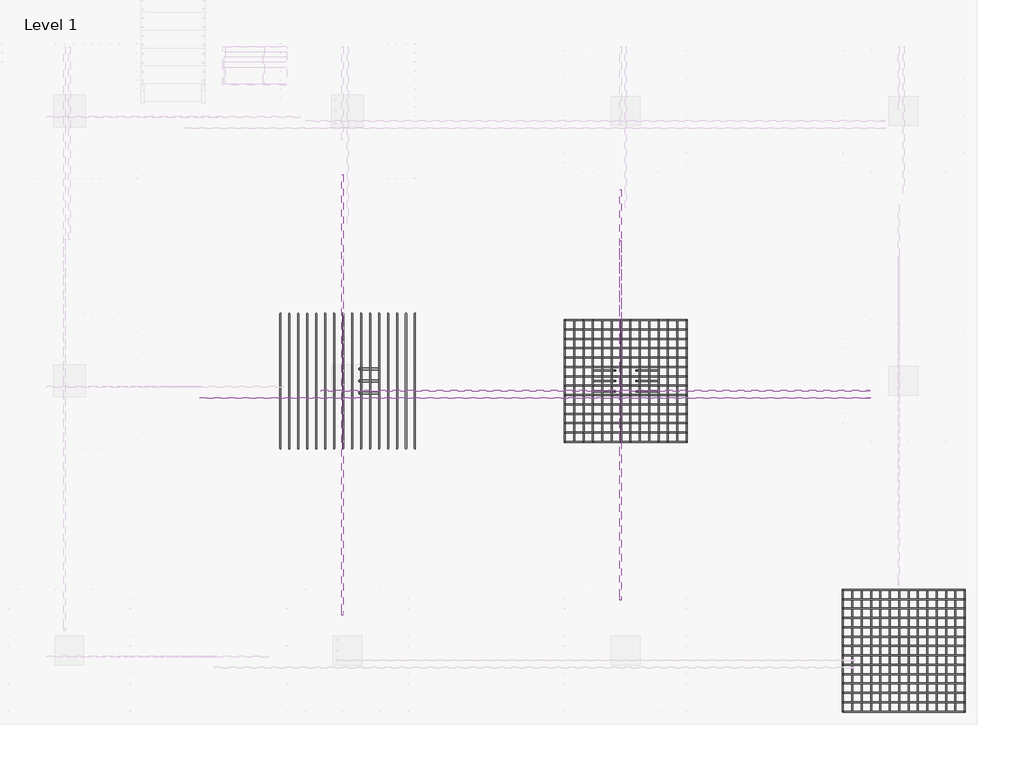
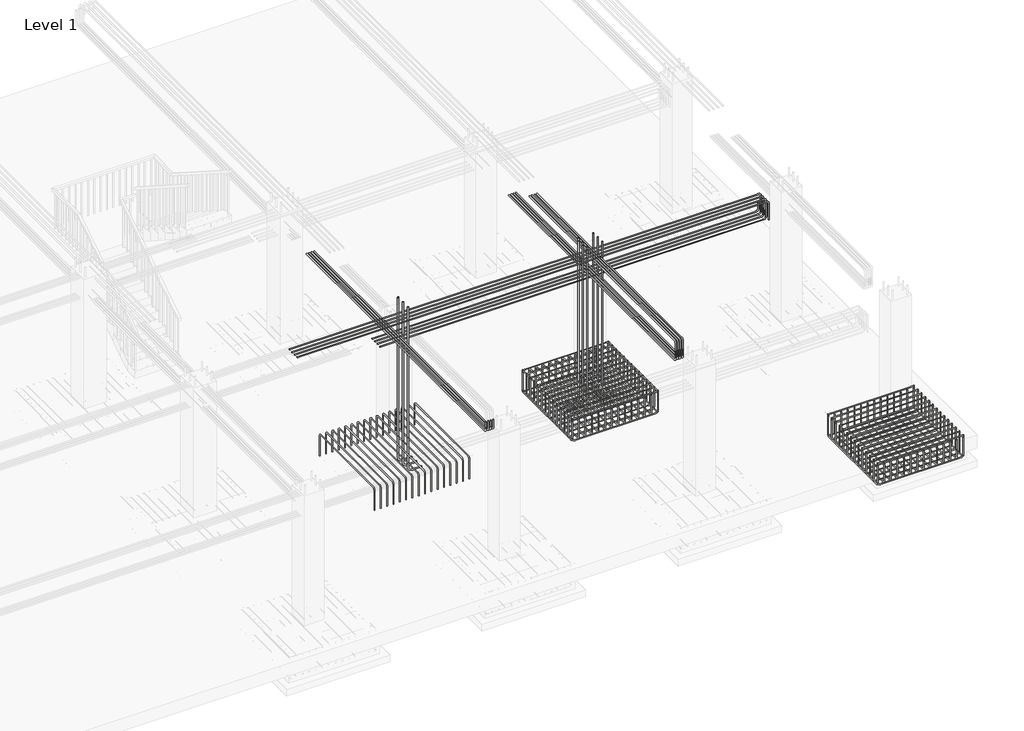
# One storey, part 7 of 17: 21 reinforcing bars.
"""IFC4 building model written with IfcOpenShell, lengths in millimetres."""

from ifc_helpers import new_model, si_unit, point, frame, origin, place, context, project, spatial, polyline, circle_curve, trimmed, segment, composite_curve, source, transform, mapped, element, save
from ifc_brep_helpers import swept_disk

model = new_model("IFC4")

# Units and contexts
model_context = context("Model", 3, world=origin())
ifc_project = project(units=[si_unit("LENGTHUNIT", "METRE", prefix="MILLI")], contexts=[model_context])

# Site, building, storey
site = spatial("IfcSite", under=ifc_project)
building = spatial("IfcBuilding", under=site)
storey = spatial("IfcBuildingStorey", under=building, Name="Level 1", Elevation=0.0)

# Reinforcing bars
placement = place(None, origin())
reinforcing_bar_shape = source(origin(), model_context, "Body", "SolidModel", [
    swept_disk(composite_curve([segment(polyline([(3693.6367997, 636.009457, -40.0), (3693.6367997, 636.009457, -504.0)]), True, "CONTINUOUS"), segment(trimmed(circle_curve(frame((3741.6367997, 636.009457, -504.0), z_axis=(0.0, -1.0, 0.0), x_axis=(-48.0, 0.0, 0.0)), 48.0), [point((3693.6367997, 636.009457, -504.0))], [point((3741.6367997, 636.009457, -552.0))], True, "CARTESIAN"), True, "CONTINUOUS"), segment(polyline([(3741.6367997, 636.009457, -552.0), (5549.6367997, 636.009457, -552.0)]), True, "CONTINUOUS"), segment(trimmed(circle_curve(frame((5549.6367997, 636.009457, -504.0), z_axis=(0.0, -1.0, 0.0), x_axis=(0.0, 0.0, -48.0)), 48.0), [point((5549.6367997, 636.009457, -552.0))], [point((5597.6367997, 636.009457, -504.0))], True, "CARTESIAN"), True, "CONTINUOUS"), segment(polyline([(5597.6367997, 636.009457, -504.0), (5597.6367997, 636.009457, -40.0)]), True, "CONTINUOUS")], self_intersect=False), 8.0),
])
element("IfcReinforcingBar", 1, at=placement, inside=storey, context=model_context, shape_type="MappedRepresentation", body=[
    mapped(reinforcing_bar_shape, transform((0.0, 0.0, 0.0), x_axis=(1.0, 0.0, 0.0), y_axis=(0.0, 1.0, 0.0), z_axis=(0.0, 0.0, 1.0))),
    mapped(reinforcing_bar_shape, transform((0.0, -146.4615385, 0.0), x_axis=(1.0, 0.0, 0.0), y_axis=(0.0, 1.0, 0.0), z_axis=(0.0, 0.0, 1.0))),
    mapped(reinforcing_bar_shape, transform((0.0, -292.9230769, 0.0), x_axis=(1.0, 0.0, 0.0), y_axis=(0.0, 1.0, 0.0), z_axis=(0.0, 0.0, 1.0))),
    mapped(reinforcing_bar_shape, transform((0.0, -439.3846154, 0.0), x_axis=(1.0, 0.0, 0.0), y_axis=(0.0, 1.0, 0.0), z_axis=(0.0, 0.0, 1.0))),
    mapped(reinforcing_bar_shape, transform((0.0, -585.8461538, 0.0), x_axis=(1.0, 0.0, 0.0), y_axis=(0.0, 1.0, 0.0), z_axis=(0.0, 0.0, 1.0))),
    mapped(reinforcing_bar_shape, transform((0.0, -732.3076923, 0.0), x_axis=(1.0, 0.0, 0.0), y_axis=(0.0, 1.0, 0.0), z_axis=(0.0, 0.0, 1.0))),
    mapped(reinforcing_bar_shape, transform((0.0, -878.7692308, 0.0), x_axis=(1.0, 0.0, 0.0), y_axis=(0.0, 1.0, 0.0), z_axis=(0.0, 0.0, 1.0))),
    mapped(reinforcing_bar_shape, transform((0.0, -1025.2307692, 0.0), x_axis=(1.0, 0.0, 0.0), y_axis=(0.0, 1.0, 0.0), z_axis=(0.0, 0.0, 1.0))),
    mapped(reinforcing_bar_shape, transform((0.0, -1171.6923077, 0.0), x_axis=(1.0, 0.0, 0.0), y_axis=(0.0, 1.0, 0.0), z_axis=(0.0, 0.0, 1.0))),
    mapped(reinforcing_bar_shape, transform((0.0, -1318.1538462, 0.0), x_axis=(1.0, 0.0, 0.0), y_axis=(0.0, 1.0, 0.0), z_axis=(0.0, 0.0, 1.0))),
    mapped(reinforcing_bar_shape, transform((0.0, -1464.6153846, 0.0), x_axis=(1.0, 0.0, 0.0), y_axis=(0.0, 1.0, 0.0), z_axis=(0.0, 0.0, 1.0))),
    mapped(reinforcing_bar_shape, transform((0.0, -1611.0769231, 0.0), x_axis=(1.0, 0.0, 0.0), y_axis=(0.0, 1.0, 0.0), z_axis=(0.0, 0.0, 1.0))),
    mapped(reinforcing_bar_shape, transform((0.0, -1757.5384615, 0.0), x_axis=(1.0, 0.0, 0.0), y_axis=(0.0, 1.0, 0.0), z_axis=(0.0, 0.0, 1.0))),
    mapped(reinforcing_bar_shape, transform((0.0, -1904.0, 0.0), x_axis=(1.0, 0.0, 0.0), y_axis=(0.0, 1.0, 0.0), z_axis=(0.0, 0.0, 1.0))),
])
reinforcing_bar_2_shape = source(origin(), model_context, "Body", "SolidModel", [
    swept_disk(composite_curve([segment(polyline([(3693.6367997, -1267.990543, -504.0), (3693.6367997, -1267.990543, -96.0)]), True, "CONTINUOUS"), segment(trimmed(circle_curve(frame((3741.6367997, -1267.990543, -96.0), z_axis=(0.0, 1.0, 0.0), x_axis=(-48.0, 0.0, 0.0)), 48.0), [point((3693.6367997, -1267.990543, -96.0))], [point((3741.6367997, -1267.990543, -48.0))], True, "CARTESIAN"), True, "CONTINUOUS"), segment(polyline([(3741.6367997, -1267.990543, -48.0), (5549.6367997, -1267.990543, -48.0)]), True, "CONTINUOUS"), segment(trimmed(circle_curve(frame((5549.6367997, -1267.990543, -96.0), z_axis=(0.0, 1.0, 0.0), x_axis=(0.0, 0.0, 48.0)), 48.0), [point((5549.6367997, -1267.990543, -48.0))], [point((5597.6367997, -1267.990543, -96.0))], True, "CARTESIAN"), True, "CONTINUOUS"), segment(polyline([(5597.6367997, -1267.990543, -96.0), (5597.6367997, -1267.990543, -504.0)]), True, "CONTINUOUS")], self_intersect=False), 8.0),
])
element("IfcReinforcingBar", 2, at=placement, inside=storey, context=model_context, shape_type="MappedRepresentation", body=[
    mapped(reinforcing_bar_2_shape, transform((0.0, 0.0, 0.0), x_axis=(1.0, 0.0, 0.0), y_axis=(0.0, 1.0, 0.0), z_axis=(0.0, 0.0, 1.0))),
    mapped(reinforcing_bar_2_shape, transform((0.0, 146.4615385, 0.0), x_axis=(1.0, 0.0, 0.0), y_axis=(0.0, 1.0, 0.0), z_axis=(0.0, 0.0, 1.0))),
    mapped(reinforcing_bar_2_shape, transform((0.0, 292.9230769, 0.0), x_axis=(1.0, 0.0, 0.0), y_axis=(0.0, 1.0, 0.0), z_axis=(0.0, 0.0, 1.0))),
    mapped(reinforcing_bar_2_shape, transform((0.0, 439.3846154, 0.0), x_axis=(1.0, 0.0, 0.0), y_axis=(0.0, 1.0, 0.0), z_axis=(0.0, 0.0, 1.0))),
    mapped(reinforcing_bar_2_shape, transform((0.0, 585.8461538, 0.0), x_axis=(1.0, 0.0, 0.0), y_axis=(0.0, 1.0, 0.0), z_axis=(0.0, 0.0, 1.0))),
    mapped(reinforcing_bar_2_shape, transform((0.0, 732.3076923, 0.0), x_axis=(1.0, 0.0, 0.0), y_axis=(0.0, 1.0, 0.0), z_axis=(0.0, 0.0, 1.0))),
    mapped(reinforcing_bar_2_shape, transform((0.0, 878.7692308, 0.0), x_axis=(1.0, 0.0, 0.0), y_axis=(0.0, 1.0, 0.0), z_axis=(0.0, 0.0, 1.0))),
    mapped(reinforcing_bar_2_shape, transform((0.0, 1025.2307692, 0.0), x_axis=(1.0, 0.0, 0.0), y_axis=(0.0, 1.0, 0.0), z_axis=(0.0, 0.0, 1.0))),
    mapped(reinforcing_bar_2_shape, transform((0.0, 1171.6923077, 0.0), x_axis=(1.0, 0.0, 0.0), y_axis=(0.0, 1.0, 0.0), z_axis=(0.0, 0.0, 1.0))),
    mapped(reinforcing_bar_2_shape, transform((0.0, 1318.1538462, 0.0), x_axis=(1.0, 0.0, 0.0), y_axis=(0.0, 1.0, 0.0), z_axis=(0.0, 0.0, 1.0))),
    mapped(reinforcing_bar_2_shape, transform((0.0, 1464.6153846, 0.0), x_axis=(1.0, 0.0, 0.0), y_axis=(0.0, 1.0, 0.0), z_axis=(0.0, 0.0, 1.0))),
    mapped(reinforcing_bar_2_shape, transform((0.0, 1611.0769231, 0.0), x_axis=(1.0, 0.0, 0.0), y_axis=(0.0, 1.0, 0.0), z_axis=(0.0, 0.0, 1.0))),
    mapped(reinforcing_bar_2_shape, transform((0.0, 1757.5384615, 0.0), x_axis=(1.0, 0.0, 0.0), y_axis=(0.0, 1.0, 0.0), z_axis=(0.0, 0.0, 1.0))),
    mapped(reinforcing_bar_2_shape, transform((0.0, 1904.0, 0.0), x_axis=(1.0, 0.0, 0.0), y_axis=(0.0, 1.0, 0.0), z_axis=(0.0, 0.0, 1.0))),
])
reinforcing_bar_3_shape = source(origin(), model_context, "Body", "SolidModel", [
    swept_disk(composite_curve([segment(polyline([(5597.6367997, 636.009457, -96.0), (5597.6367997, 636.009457, -504.0)]), True, "CONTINUOUS"), segment(trimmed(circle_curve(frame((5597.6367997, 588.009457, -504.0), z_axis=(-1.0, 0.0, 0.0), x_axis=(0.0, 48.0, 0.0)), 48.0), [point((5597.6367997, 636.009457, -504.0))], [point((5597.6367997, 588.009457, -552.0))], True, "CARTESIAN"), True, "CONTINUOUS"), segment(polyline([(5597.6367997, 588.009457, -552.0), (5597.6367997, -1219.990543, -552.0)]), True, "CONTINUOUS"), segment(trimmed(circle_curve(frame((5597.6367997, -1219.990543, -504.0), z_axis=(-1.0, 0.0, 0.0), x_axis=(0.0, 0.0, -48.0)), 48.0), [point((5597.6367997, -1219.990543, -552.0))], [point((5597.6367997, -1267.990543, -504.0))], True, "CARTESIAN"), True, "CONTINUOUS"), segment(polyline([(5597.6367997, -1267.990543, -504.0), (5597.6367997, -1267.990543, -96.0)]), True, "CONTINUOUS")], self_intersect=False), 8.0),
])
element("IfcReinforcingBar", 3, at=placement, inside=storey, context=model_context, shape_type="MappedRepresentation", body=[
    mapped(reinforcing_bar_3_shape, transform((0.0, 0.0, 0.0), x_axis=(1.0, 0.0, 0.0), y_axis=(0.0, 1.0, 0.0), z_axis=(0.0, 0.0, 1.0))),
    mapped(reinforcing_bar_3_shape, transform((-146.4615385, 0.0, 0.0), x_axis=(1.0, 0.0, 0.0), y_axis=(0.0, 1.0, 0.0), z_axis=(0.0, 0.0, 1.0))),
    mapped(reinforcing_bar_3_shape, transform((-292.9230769, 0.0, 0.0), x_axis=(1.0, 0.0, 0.0), y_axis=(0.0, 1.0, 0.0), z_axis=(0.0, 0.0, 1.0))),
    mapped(reinforcing_bar_3_shape, transform((-439.3846154, 0.0, 0.0), x_axis=(1.0, 0.0, 0.0), y_axis=(0.0, 1.0, 0.0), z_axis=(0.0, 0.0, 1.0))),
    mapped(reinforcing_bar_3_shape, transform((-585.8461538, 0.0, 0.0), x_axis=(1.0, 0.0, 0.0), y_axis=(0.0, 1.0, 0.0), z_axis=(0.0, 0.0, 1.0))),
    mapped(reinforcing_bar_3_shape, transform((-732.3076923, 0.0, 0.0), x_axis=(1.0, 0.0, 0.0), y_axis=(0.0, 1.0, 0.0), z_axis=(0.0, 0.0, 1.0))),
    mapped(reinforcing_bar_3_shape, transform((-878.7692308, 0.0, 0.0), x_axis=(1.0, 0.0, 0.0), y_axis=(0.0, 1.0, 0.0), z_axis=(0.0, 0.0, 1.0))),
    mapped(reinforcing_bar_3_shape, transform((-1025.2307692, 0.0, 0.0), x_axis=(1.0, 0.0, 0.0), y_axis=(0.0, 1.0, 0.0), z_axis=(0.0, 0.0, 1.0))),
    mapped(reinforcing_bar_3_shape, transform((-1171.6923077, 0.0, 0.0), x_axis=(1.0, 0.0, 0.0), y_axis=(0.0, 1.0, 0.0), z_axis=(0.0, 0.0, 1.0))),
    mapped(reinforcing_bar_3_shape, transform((-1318.1538462, 0.0, 0.0), x_axis=(1.0, 0.0, 0.0), y_axis=(0.0, 1.0, 0.0), z_axis=(0.0, 0.0, 1.0))),
    mapped(reinforcing_bar_3_shape, transform((-1464.6153846, 0.0, 0.0), x_axis=(1.0, 0.0, 0.0), y_axis=(0.0, 1.0, 0.0), z_axis=(0.0, 0.0, 1.0))),
    mapped(reinforcing_bar_3_shape, transform((-1611.0769231, 0.0, 0.0), x_axis=(1.0, 0.0, 0.0), y_axis=(0.0, 1.0, 0.0), z_axis=(0.0, 0.0, 1.0))),
    mapped(reinforcing_bar_3_shape, transform((-1757.5384615, 0.0, 0.0), x_axis=(1.0, 0.0, 0.0), y_axis=(0.0, 1.0, 0.0), z_axis=(0.0, 0.0, 1.0))),
    mapped(reinforcing_bar_3_shape, transform((-1904.0, 0.0, 0.0), x_axis=(1.0, 0.0, 0.0), y_axis=(0.0, 1.0, 0.0), z_axis=(0.0, 0.0, 1.0))),
])
reinforcing_bar_4_shape = source(origin(), model_context, "Body", "SolidModel", [
    swept_disk(composite_curve([segment(polyline([(3693.6367997, 636.009457, -504.0), (3693.6367997, 636.009457, -96.0)]), True, "CONTINUOUS"), segment(trimmed(circle_curve(frame((3693.6367997, 588.009457, -96.0), z_axis=(1.0, 0.0, 0.0), x_axis=(0.0, 48.0, 0.0)), 48.0), [point((3693.6367997, 636.009457, -96.0))], [point((3693.6367997, 588.009457, -48.0))], True, "CARTESIAN"), True, "CONTINUOUS"), segment(polyline([(3693.6367997, 588.009457, -48.0), (3693.6367997, -1219.990543, -48.0)]), True, "CONTINUOUS"), segment(trimmed(circle_curve(frame((3693.6367997, -1219.990543, -96.0), z_axis=(1.0, 0.0, 0.0), x_axis=(0.0, 0.0, 48.0)), 48.0), [point((3693.6367997, -1219.990543, -48.0))], [point((3693.6367997, -1267.990543, -96.0))], True, "CARTESIAN"), True, "CONTINUOUS"), segment(polyline([(3693.6367997, -1267.990543, -96.0), (3693.6367997, -1267.990543, -504.0)]), True, "CONTINUOUS")], self_intersect=False), 8.0),
])
element("IfcReinforcingBar", 4, at=placement, inside=storey, context=model_context, shape_type="MappedRepresentation", body=[
    mapped(reinforcing_bar_4_shape, transform((0.0, 0.0, 0.0), x_axis=(1.0, 0.0, 0.0), y_axis=(0.0, 1.0, 0.0), z_axis=(0.0, 0.0, 1.0))),
    mapped(reinforcing_bar_4_shape, transform((146.4615385, 0.0, 0.0), x_axis=(1.0, 0.0, 0.0), y_axis=(0.0, 1.0, 0.0), z_axis=(0.0, 0.0, 1.0))),
    mapped(reinforcing_bar_4_shape, transform((292.9230769, 0.0, 0.0), x_axis=(1.0, 0.0, 0.0), y_axis=(0.0, 1.0, 0.0), z_axis=(0.0, 0.0, 1.0))),
    mapped(reinforcing_bar_4_shape, transform((439.3846154, 0.0, 0.0), x_axis=(1.0, 0.0, 0.0), y_axis=(0.0, 1.0, 0.0), z_axis=(0.0, 0.0, 1.0))),
    mapped(reinforcing_bar_4_shape, transform((585.8461538, 0.0, 0.0), x_axis=(1.0, 0.0, 0.0), y_axis=(0.0, 1.0, 0.0), z_axis=(0.0, 0.0, 1.0))),
    mapped(reinforcing_bar_4_shape, transform((732.3076923, 0.0, 0.0), x_axis=(1.0, 0.0, 0.0), y_axis=(0.0, 1.0, 0.0), z_axis=(0.0, 0.0, 1.0))),
    mapped(reinforcing_bar_4_shape, transform((878.7692308, 0.0, 0.0), x_axis=(1.0, 0.0, 0.0), y_axis=(0.0, 1.0, 0.0), z_axis=(0.0, 0.0, 1.0))),
    mapped(reinforcing_bar_4_shape, transform((1025.2307692, 0.0, 0.0), x_axis=(1.0, 0.0, 0.0), y_axis=(0.0, 1.0, 0.0), z_axis=(0.0, 0.0, 1.0))),
    mapped(reinforcing_bar_4_shape, transform((1171.6923077, 0.0, 0.0), x_axis=(1.0, 0.0, 0.0), y_axis=(0.0, 1.0, 0.0), z_axis=(0.0, 0.0, 1.0))),
    mapped(reinforcing_bar_4_shape, transform((1318.1538462, 0.0, 0.0), x_axis=(1.0, 0.0, 0.0), y_axis=(0.0, 1.0, 0.0), z_axis=(0.0, 0.0, 1.0))),
    mapped(reinforcing_bar_4_shape, transform((1464.6153846, 0.0, 0.0), x_axis=(1.0, 0.0, 0.0), y_axis=(0.0, 1.0, 0.0), z_axis=(0.0, 0.0, 1.0))),
    mapped(reinforcing_bar_4_shape, transform((1611.0769231, 0.0, 0.0), x_axis=(1.0, 0.0, 0.0), y_axis=(0.0, 1.0, 0.0), z_axis=(0.0, 0.0, 1.0))),
    mapped(reinforcing_bar_4_shape, transform((1757.5384615, 0.0, 0.0), x_axis=(1.0, 0.0, 0.0), y_axis=(0.0, 1.0, 0.0), z_axis=(0.0, 0.0, 1.0))),
    mapped(reinforcing_bar_4_shape, transform((1904.0, 0.0, 0.0), x_axis=(1.0, 0.0, 0.0), y_axis=(0.0, 1.0, 0.0), z_axis=(0.0, 0.0, 1.0))),
])
reinforcing_bar_5_shape = source(origin(), model_context, "Body", "SolidModel", [
    swept_disk(composite_curve([segment(polyline([(4133.0214151, -150.490543, -550.0), (4430.1367997, -150.490543, -550.0)]), True, "CONTINUOUS"), segment(trimmed(circle_curve(frame((4430.1367997, -150.490543, -500.0), z_axis=(0.0, -1.0, 0.0), x_axis=(0.0, 0.0, -50.0)), 50.0), [point((4430.1367997, -150.490543, -550.0))], [point((4480.1367997, -150.490543, -500.0))], True, "CARTESIAN"), True, "CONTINUOUS"), segment(polyline([(4480.1367997, -150.490543, -500.0), (4480.1367997, -150.490543, 3260.0)]), True, "CONTINUOUS")], self_intersect=False), 10.0),
])
element("IfcReinforcingBar", 5, at=placement, inside=storey, context=model_context, shape_type="MappedRepresentation", body=[
    mapped(reinforcing_bar_5_shape, transform((0.0, 0.0, 0.0), x_axis=(1.0, 0.0, 0.0), y_axis=(0.0, 1.0, 0.0), z_axis=(0.0, 0.0, 1.0))),
    mapped(reinforcing_bar_5_shape, transform((0.0, -165.5, 0.0), x_axis=(1.0, 0.0, 0.0), y_axis=(0.0, 1.0, 0.0), z_axis=(0.0, 0.0, 1.0))),
    mapped(reinforcing_bar_5_shape, transform((0.0, -331.0, 0.0), x_axis=(1.0, 0.0, 0.0), y_axis=(0.0, 1.0, 0.0), z_axis=(0.0, 0.0, 1.0))),
])
reinforcing_bar_6_shape = source(origin(), model_context, "Body", "SolidModel", [
    swept_disk(composite_curve([segment(polyline([(5158.2521843, -481.490543, -550.0), (4861.1367997, -481.490543, -550.0)]), True, "CONTINUOUS"), segment(trimmed(circle_curve(frame((4861.1367997, -481.490543, -500.0), z_axis=(0.0, 1.0, 0.0), x_axis=(0.0, 0.0, -50.0)), 50.0), [point((4861.1367997, -481.490543, -550.0))], [point((4811.1367997, -481.490543, -500.0))], True, "CARTESIAN"), True, "CONTINUOUS"), segment(polyline([(4811.1367997, -481.490543, -500.0), (4811.1367997, -481.490543, 3260.0)]), True, "CONTINUOUS")], self_intersect=False), 10.0),
])
element("IfcReinforcingBar", 6, at=placement, inside=storey, context=model_context, shape_type="MappedRepresentation", body=[
    mapped(reinforcing_bar_6_shape, transform((0.0, 0.0, 0.0), x_axis=(1.0, 0.0, 0.0), y_axis=(0.0, 1.0, 0.0), z_axis=(0.0, 0.0, 1.0))),
    mapped(reinforcing_bar_6_shape, transform((0.0, 165.5, 0.0), x_axis=(1.0, 0.0, 0.0), y_axis=(0.0, 1.0, 0.0), z_axis=(0.0, 0.0, 1.0))),
    mapped(reinforcing_bar_6_shape, transform((0.0, 331.0, 0.0), x_axis=(1.0, 0.0, 0.0), y_axis=(0.0, 1.0, 0.0), z_axis=(0.0, 0.0, 1.0))),
])
reinforcing_bar_7_shape = source(origin(), model_context, "Body", "SolidModel", [
    swept_disk(composite_curve([segment(polyline([(8038.6367997, -3580.990543, -40.0), (8038.6367997, -3580.990543, -504.0)]), True, "CONTINUOUS"), segment(trimmed(circle_curve(frame((8086.6367997, -3580.990543, -504.0), z_axis=(0.0, -1.0, 0.0), x_axis=(-48.0, 0.0, 0.0)), 48.0), [point((8038.6367997, -3580.990543, -504.0))], [point((8086.6367997, -3580.990543, -552.0))], True, "CARTESIAN"), True, "CONTINUOUS"), segment(polyline([(8086.6367997, -3580.990543, -552.0), (9894.6367997, -3580.990543, -552.0)]), True, "CONTINUOUS"), segment(trimmed(circle_curve(frame((9894.6367997, -3580.990543, -504.0), z_axis=(0.0, -1.0, 0.0), x_axis=(0.0, 0.0, -48.0)), 48.0), [point((9894.6367997, -3580.990543, -552.0))], [point((9942.6367997, -3580.990543, -504.0))], True, "CARTESIAN"), True, "CONTINUOUS"), segment(polyline([(9942.6367997, -3580.990543, -504.0), (9942.6367997, -3580.990543, -40.0)]), True, "CONTINUOUS")], self_intersect=False), 8.0),
])
element("IfcReinforcingBar", 7, at=placement, inside=storey, context=model_context, shape_type="MappedRepresentation", body=[
    mapped(reinforcing_bar_7_shape, transform((0.0, 0.0, 0.0), x_axis=(1.0, 0.0, 0.0), y_axis=(0.0, 1.0, 0.0), z_axis=(0.0, 0.0, 1.0))),
    mapped(reinforcing_bar_7_shape, transform((0.0, -146.4615385, 0.0), x_axis=(1.0, 0.0, 0.0), y_axis=(0.0, 1.0, 0.0), z_axis=(0.0, 0.0, 1.0))),
    mapped(reinforcing_bar_7_shape, transform((0.0, -292.9230769, 0.0), x_axis=(1.0, 0.0, 0.0), y_axis=(0.0, 1.0, 0.0), z_axis=(0.0, 0.0, 1.0))),
    mapped(reinforcing_bar_7_shape, transform((0.0, -439.3846154, 0.0), x_axis=(1.0, 0.0, 0.0), y_axis=(0.0, 1.0, 0.0), z_axis=(0.0, 0.0, 1.0))),
    mapped(reinforcing_bar_7_shape, transform((0.0, -585.8461538, 0.0), x_axis=(1.0, 0.0, 0.0), y_axis=(0.0, 1.0, 0.0), z_axis=(0.0, 0.0, 1.0))),
    mapped(reinforcing_bar_7_shape, transform((0.0, -732.3076923, 0.0), x_axis=(1.0, 0.0, 0.0), y_axis=(0.0, 1.0, 0.0), z_axis=(0.0, 0.0, 1.0))),
    mapped(reinforcing_bar_7_shape, transform((0.0, -878.7692308, 0.0), x_axis=(1.0, 0.0, 0.0), y_axis=(0.0, 1.0, 0.0), z_axis=(0.0, 0.0, 1.0))),
    mapped(reinforcing_bar_7_shape, transform((0.0, -1025.2307692, 0.0), x_axis=(1.0, 0.0, 0.0), y_axis=(0.0, 1.0, 0.0), z_axis=(0.0, 0.0, 1.0))),
    mapped(reinforcing_bar_7_shape, transform((0.0, -1171.6923077, 0.0), x_axis=(1.0, 0.0, 0.0), y_axis=(0.0, 1.0, 0.0), z_axis=(0.0, 0.0, 1.0))),
    mapped(reinforcing_bar_7_shape, transform((0.0, -1318.1538462, 0.0), x_axis=(1.0, 0.0, 0.0), y_axis=(0.0, 1.0, 0.0), z_axis=(0.0, 0.0, 1.0))),
    mapped(reinforcing_bar_7_shape, transform((0.0, -1464.6153846, 0.0), x_axis=(1.0, 0.0, 0.0), y_axis=(0.0, 1.0, 0.0), z_axis=(0.0, 0.0, 1.0))),
    mapped(reinforcing_bar_7_shape, transform((0.0, -1611.0769231, 0.0), x_axis=(1.0, 0.0, 0.0), y_axis=(0.0, 1.0, 0.0), z_axis=(0.0, 0.0, 1.0))),
    mapped(reinforcing_bar_7_shape, transform((0.0, -1757.5384615, 0.0), x_axis=(1.0, 0.0, 0.0), y_axis=(0.0, 1.0, 0.0), z_axis=(0.0, 0.0, 1.0))),
    mapped(reinforcing_bar_7_shape, transform((0.0, -1904.0, 0.0), x_axis=(1.0, 0.0, 0.0), y_axis=(0.0, 1.0, 0.0), z_axis=(0.0, 0.0, 1.0))),
])
reinforcing_bar_8_shape = source(origin(), model_context, "Body", "SolidModel", [
    swept_disk(composite_curve([segment(polyline([(8038.6367997, -5484.990543, -504.0), (8038.6367997, -5484.990543, -96.0)]), True, "CONTINUOUS"), segment(trimmed(circle_curve(frame((8086.6367997, -5484.990543, -96.0), z_axis=(0.0, 1.0, 0.0), x_axis=(-48.0, 0.0, 0.0)), 48.0), [point((8038.6367997, -5484.990543, -96.0))], [point((8086.6367997, -5484.990543, -48.0))], True, "CARTESIAN"), True, "CONTINUOUS"), segment(polyline([(8086.6367997, -5484.990543, -48.0), (9894.6367997, -5484.990543, -48.0)]), True, "CONTINUOUS"), segment(trimmed(circle_curve(frame((9894.6367997, -5484.990543, -96.0), z_axis=(0.0, 1.0, 0.0), x_axis=(0.0, 0.0, 48.0)), 48.0), [point((9894.6367997, -5484.990543, -48.0))], [point((9942.6367997, -5484.990543, -96.0))], True, "CARTESIAN"), True, "CONTINUOUS"), segment(polyline([(9942.6367997, -5484.990543, -96.0), (9942.6367997, -5484.990543, -504.0)]), True, "CONTINUOUS")], self_intersect=False), 8.0),
])
element("IfcReinforcingBar", 8, at=placement, inside=storey, context=model_context, shape_type="MappedRepresentation", body=[
    mapped(reinforcing_bar_8_shape, transform((0.0, 0.0, 0.0), x_axis=(1.0, 0.0, 0.0), y_axis=(0.0, 1.0, 0.0), z_axis=(0.0, 0.0, 1.0))),
    mapped(reinforcing_bar_8_shape, transform((0.0, 146.4615385, 0.0), x_axis=(1.0, 0.0, 0.0), y_axis=(0.0, 1.0, 0.0), z_axis=(0.0, 0.0, 1.0))),
    mapped(reinforcing_bar_8_shape, transform((0.0, 292.9230769, 0.0), x_axis=(1.0, 0.0, 0.0), y_axis=(0.0, 1.0, 0.0), z_axis=(0.0, 0.0, 1.0))),
    mapped(reinforcing_bar_8_shape, transform((0.0, 439.3846154, 0.0), x_axis=(1.0, 0.0, 0.0), y_axis=(0.0, 1.0, 0.0), z_axis=(0.0, 0.0, 1.0))),
    mapped(reinforcing_bar_8_shape, transform((0.0, 585.8461538, 0.0), x_axis=(1.0, 0.0, 0.0), y_axis=(0.0, 1.0, 0.0), z_axis=(0.0, 0.0, 1.0))),
    mapped(reinforcing_bar_8_shape, transform((0.0, 732.3076923, 0.0), x_axis=(1.0, 0.0, 0.0), y_axis=(0.0, 1.0, 0.0), z_axis=(0.0, 0.0, 1.0))),
    mapped(reinforcing_bar_8_shape, transform((0.0, 878.7692308, 0.0), x_axis=(1.0, 0.0, 0.0), y_axis=(0.0, 1.0, 0.0), z_axis=(0.0, 0.0, 1.0))),
    mapped(reinforcing_bar_8_shape, transform((0.0, 1025.2307692, 0.0), x_axis=(1.0, 0.0, 0.0), y_axis=(0.0, 1.0, 0.0), z_axis=(0.0, 0.0, 1.0))),
    mapped(reinforcing_bar_8_shape, transform((0.0, 1171.6923077, 0.0), x_axis=(1.0, 0.0, 0.0), y_axis=(0.0, 1.0, 0.0), z_axis=(0.0, 0.0, 1.0))),
    mapped(reinforcing_bar_8_shape, transform((0.0, 1318.1538462, 0.0), x_axis=(1.0, 0.0, 0.0), y_axis=(0.0, 1.0, 0.0), z_axis=(0.0, 0.0, 1.0))),
    mapped(reinforcing_bar_8_shape, transform((0.0, 1464.6153846, 0.0), x_axis=(1.0, 0.0, 0.0), y_axis=(0.0, 1.0, 0.0), z_axis=(0.0, 0.0, 1.0))),
    mapped(reinforcing_bar_8_shape, transform((0.0, 1611.0769231, 0.0), x_axis=(1.0, 0.0, 0.0), y_axis=(0.0, 1.0, 0.0), z_axis=(0.0, 0.0, 1.0))),
    mapped(reinforcing_bar_8_shape, transform((0.0, 1757.5384615, 0.0), x_axis=(1.0, 0.0, 0.0), y_axis=(0.0, 1.0, 0.0), z_axis=(0.0, 0.0, 1.0))),
    mapped(reinforcing_bar_8_shape, transform((0.0, 1904.0, 0.0), x_axis=(1.0, 0.0, 0.0), y_axis=(0.0, 1.0, 0.0), z_axis=(0.0, 0.0, 1.0))),
])
reinforcing_bar_9_shape = source(origin(), model_context, "Body", "SolidModel", [
    swept_disk(composite_curve([segment(polyline([(9942.6367997, -3580.990543, -96.0), (9942.6367997, -3580.990543, -504.0)]), True, "CONTINUOUS"), segment(trimmed(circle_curve(frame((9942.6367997, -3628.990543, -504.0), z_axis=(-1.0, 0.0, 0.0), x_axis=(0.0, 48.0, 0.0)), 48.0), [point((9942.6367997, -3580.990543, -504.0))], [point((9942.6367997, -3628.990543, -552.0))], True, "CARTESIAN"), True, "CONTINUOUS"), segment(polyline([(9942.6367997, -3628.990543, -552.0), (9942.6367997, -5436.990543, -552.0)]), True, "CONTINUOUS"), segment(trimmed(circle_curve(frame((9942.6367997, -5436.990543, -504.0), z_axis=(-1.0, 0.0, 0.0), x_axis=(0.0, 0.0, -48.0)), 48.0), [point((9942.6367997, -5436.990543, -552.0))], [point((9942.6367997, -5484.990543, -504.0))], True, "CARTESIAN"), True, "CONTINUOUS"), segment(polyline([(9942.6367997, -5484.990543, -504.0), (9942.6367997, -5484.990543, -96.0)]), True, "CONTINUOUS")], self_intersect=False), 8.0),
])
element("IfcReinforcingBar", 9, at=placement, inside=storey, context=model_context, shape_type="MappedRepresentation", body=[
    mapped(reinforcing_bar_9_shape, transform((0.0, 0.0, 0.0), x_axis=(1.0, 0.0, 0.0), y_axis=(0.0, 1.0, 0.0), z_axis=(0.0, 0.0, 1.0))),
    mapped(reinforcing_bar_9_shape, transform((-146.4615385, 0.0, 0.0), x_axis=(1.0, 0.0, 0.0), y_axis=(0.0, 1.0, 0.0), z_axis=(0.0, 0.0, 1.0))),
    mapped(reinforcing_bar_9_shape, transform((-292.9230769, 0.0, 0.0), x_axis=(1.0, 0.0, 0.0), y_axis=(0.0, 1.0, 0.0), z_axis=(0.0, 0.0, 1.0))),
    mapped(reinforcing_bar_9_shape, transform((-439.3846154, 0.0, 0.0), x_axis=(1.0, 0.0, 0.0), y_axis=(0.0, 1.0, 0.0), z_axis=(0.0, 0.0, 1.0))),
    mapped(reinforcing_bar_9_shape, transform((-585.8461538, 0.0, 0.0), x_axis=(1.0, 0.0, 0.0), y_axis=(0.0, 1.0, 0.0), z_axis=(0.0, 0.0, 1.0))),
    mapped(reinforcing_bar_9_shape, transform((-732.3076923, 0.0, 0.0), x_axis=(1.0, 0.0, 0.0), y_axis=(0.0, 1.0, 0.0), z_axis=(0.0, 0.0, 1.0))),
    mapped(reinforcing_bar_9_shape, transform((-878.7692308, 0.0, 0.0), x_axis=(1.0, 0.0, 0.0), y_axis=(0.0, 1.0, 0.0), z_axis=(0.0, 0.0, 1.0))),
    mapped(reinforcing_bar_9_shape, transform((-1025.2307692, 0.0, 0.0), x_axis=(1.0, 0.0, 0.0), y_axis=(0.0, 1.0, 0.0), z_axis=(0.0, 0.0, 1.0))),
    mapped(reinforcing_bar_9_shape, transform((-1171.6923077, 0.0, 0.0), x_axis=(1.0, 0.0, 0.0), y_axis=(0.0, 1.0, 0.0), z_axis=(0.0, 0.0, 1.0))),
    mapped(reinforcing_bar_9_shape, transform((-1318.1538462, 0.0, 0.0), x_axis=(1.0, 0.0, 0.0), y_axis=(0.0, 1.0, 0.0), z_axis=(0.0, 0.0, 1.0))),
    mapped(reinforcing_bar_9_shape, transform((-1464.6153846, 0.0, 0.0), x_axis=(1.0, 0.0, 0.0), y_axis=(0.0, 1.0, 0.0), z_axis=(0.0, 0.0, 1.0))),
    mapped(reinforcing_bar_9_shape, transform((-1611.0769231, 0.0, 0.0), x_axis=(1.0, 0.0, 0.0), y_axis=(0.0, 1.0, 0.0), z_axis=(0.0, 0.0, 1.0))),
    mapped(reinforcing_bar_9_shape, transform((-1757.5384615, 0.0, 0.0), x_axis=(1.0, 0.0, 0.0), y_axis=(0.0, 1.0, 0.0), z_axis=(0.0, 0.0, 1.0))),
    mapped(reinforcing_bar_9_shape, transform((-1904.0, 0.0, 0.0), x_axis=(1.0, 0.0, 0.0), y_axis=(0.0, 1.0, 0.0), z_axis=(0.0, 0.0, 1.0))),
])
reinforcing_bar_10_shape = source(origin(), model_context, "Body", "SolidModel", [
    swept_disk(composite_curve([segment(polyline([(-751.3632003, 736.009457, -560.0), (-751.3632003, 736.009457, -96.0)]), True, "CONTINUOUS"), segment(trimmed(circle_curve(frame((-751.3632003, 688.009457, -96.0), z_axis=(1.0, 0.0, 0.0), x_axis=(0.0, 48.0, 0.0)), 48.0), [point((-751.3632003, 736.009457, -96.0))], [point((-751.3632003, 688.009457, -48.0))], True, "CARTESIAN"), True, "CONTINUOUS"), segment(polyline([(-751.3632003, 688.009457, -48.0), (-751.3632003, -1319.990543, -48.0)]), True, "CONTINUOUS"), segment(trimmed(circle_curve(frame((-751.3632003, -1319.990543, -96.0), z_axis=(1.0, 0.0, 0.0), x_axis=(0.0, 0.0, 48.0)), 48.0), [point((-751.3632003, -1319.990543, -48.0))], [point((-751.3632003, -1367.990543, -96.0))], True, "CARTESIAN"), True, "CONTINUOUS"), segment(polyline([(-751.3632003, -1367.990543, -96.0), (-751.3632003, -1367.990543, -560.0)]), True, "CONTINUOUS")], self_intersect=False), 8.0),
])
element("IfcReinforcingBar", 10, at=placement, inside=storey, context=model_context, shape_type="MappedRepresentation", body=[
    mapped(reinforcing_bar_10_shape, transform((0.0, 0.0, 0.0), x_axis=(1.0, 0.0, 0.0), y_axis=(0.0, 1.0, 0.0), z_axis=(0.0, 0.0, 1.0))),
    mapped(reinforcing_bar_10_shape, transform((140.2666667, 0.0, 0.0), x_axis=(1.0, 0.0, 0.0), y_axis=(0.0, 1.0, 0.0), z_axis=(0.0, 0.0, 1.0))),
    mapped(reinforcing_bar_10_shape, transform((280.5333333, 0.0, 0.0), x_axis=(1.0, 0.0, 0.0), y_axis=(0.0, 1.0, 0.0), z_axis=(0.0, 0.0, 1.0))),
    mapped(reinforcing_bar_10_shape, transform((420.8, 0.0, 0.0), x_axis=(1.0, 0.0, 0.0), y_axis=(0.0, 1.0, 0.0), z_axis=(0.0, 0.0, 1.0))),
    mapped(reinforcing_bar_10_shape, transform((561.0666667, 0.0, 0.0), x_axis=(1.0, 0.0, 0.0), y_axis=(0.0, 1.0, 0.0), z_axis=(0.0, 0.0, 1.0))),
    mapped(reinforcing_bar_10_shape, transform((701.3333333, 0.0, 0.0), x_axis=(1.0, 0.0, 0.0), y_axis=(0.0, 1.0, 0.0), z_axis=(0.0, 0.0, 1.0))),
    mapped(reinforcing_bar_10_shape, transform((841.6, 0.0, 0.0), x_axis=(1.0, 0.0, 0.0), y_axis=(0.0, 1.0, 0.0), z_axis=(0.0, 0.0, 1.0))),
    mapped(reinforcing_bar_10_shape, transform((981.8666667, 0.0, 0.0), x_axis=(1.0, 0.0, 0.0), y_axis=(0.0, 1.0, 0.0), z_axis=(0.0, 0.0, 1.0))),
    mapped(reinforcing_bar_10_shape, transform((1122.1333333, 0.0, 0.0), x_axis=(1.0, 0.0, 0.0), y_axis=(0.0, 1.0, 0.0), z_axis=(0.0, 0.0, 1.0))),
    mapped(reinforcing_bar_10_shape, transform((1262.4, 0.0, 0.0), x_axis=(1.0, 0.0, 0.0), y_axis=(0.0, 1.0, 0.0), z_axis=(0.0, 0.0, 1.0))),
    mapped(reinforcing_bar_10_shape, transform((1402.6666667, 0.0, 0.0), x_axis=(1.0, 0.0, 0.0), y_axis=(0.0, 1.0, 0.0), z_axis=(0.0, 0.0, 1.0))),
    mapped(reinforcing_bar_10_shape, transform((1542.9333333, 0.0, 0.0), x_axis=(1.0, 0.0, 0.0), y_axis=(0.0, 1.0, 0.0), z_axis=(0.0, 0.0, 1.0))),
    mapped(reinforcing_bar_10_shape, transform((1683.2, 0.0, 0.0), x_axis=(1.0, 0.0, 0.0), y_axis=(0.0, 1.0, 0.0), z_axis=(0.0, 0.0, 1.0))),
    mapped(reinforcing_bar_10_shape, transform((1823.4666667, 0.0, 0.0), x_axis=(1.0, 0.0, 0.0), y_axis=(0.0, 1.0, 0.0), z_axis=(0.0, 0.0, 1.0))),
    mapped(reinforcing_bar_10_shape, transform((1963.7333333, 0.0, 0.0), x_axis=(1.0, 0.0, 0.0), y_axis=(0.0, 1.0, 0.0), z_axis=(0.0, 0.0, 1.0))),
    mapped(reinforcing_bar_10_shape, transform((2104.0, 0.0, 0.0), x_axis=(1.0, 0.0, 0.0), y_axis=(0.0, 1.0, 0.0), z_axis=(0.0, 0.0, 1.0))),
])
reinforcing_bar_11_shape = source(origin(), model_context, "Body", "SolidModel", [
    swept_disk(composite_curve([segment(polyline([(791.570133, -503.790543, -597.3), (578.6367997, -503.790543, -597.3)]), True, "CONTINUOUS"), segment(trimmed(circle_curve(frame((578.6367997, -503.790543, -507.1), z_axis=(0.0, 1.0, 0.0), x_axis=(0.0, 0.0, -90.19999999999993)), 90.2), [point((578.6367997, -503.790543, -597.3))], [point((488.4367997, -503.790543, -507.1))], True, "CARTESIAN"), True, "CONTINUOUS"), segment(polyline([(488.4367997, -503.790543, -507.1), (488.4367997, -503.790543, 3250.0)]), True, "CONTINUOUS")], self_intersect=False), 12.7),
])
element("IfcReinforcingBar", 11, at=placement, inside=storey, context=model_context, shape_type="MappedRepresentation", body=[
    mapped(reinforcing_bar_11_shape, transform((0.0, 0.0, 0.0), x_axis=(1.0, 0.0, 0.0), y_axis=(0.0, 1.0, 0.0), z_axis=(0.0, 0.0, 1.0))),
    mapped(reinforcing_bar_11_shape, transform((0.0, 187.8, 0.0), x_axis=(1.0, 0.0, 0.0), y_axis=(0.0, 1.0, 0.0), z_axis=(0.0, 0.0, 1.0))),
    mapped(reinforcing_bar_11_shape, transform((0.0, 375.6, 0.0), x_axis=(1.0, 0.0, 0.0), y_axis=(0.0, 1.0, 0.0), z_axis=(0.0, 0.0, 1.0))),
])
reinforcing_bar_12_shape = source(origin(), model_context, "Body", "SolidModel", [
    swept_disk(composite_curve([segment(polyline([(8452.5367997, -466.490543, 2707.4), (8452.5367997, -466.490543, 2557.5)]), True, "CONTINUOUS"), segment(trimmed(circle_curve(frame((8402.5367997, -466.490543, 2557.5), z_axis=(0.0, 1.0, 0.0), x_axis=(50.0, 0.0, 0.0)), 50.0), [point((8452.5367997, -466.490543, 2557.5))], [point((8402.5367997, -466.490543, 2507.5))], True, "CARTESIAN"), True, "CONTINUOUS"), segment(polyline([(8402.5367997, -466.490543, 2507.5), (-111.2632003, -466.490543, 2507.5)]), True, "CONTINUOUS")], self_intersect=False), 10.0),
])
element("IfcReinforcingBar", 12, at=placement, inside=storey, context=model_context, shape_type="MappedRepresentation", body=[
    mapped(reinforcing_bar_12_shape, transform((0.0, 0.0, 0.0), x_axis=(1.0, 0.0, 0.0), y_axis=(0.0, 1.0, 0.0), z_axis=(0.0, 0.0, 1.0))),
    mapped(reinforcing_bar_12_shape, transform((0.0, 98.4333333, 0.0), x_axis=(1.0, 0.0, 0.0), y_axis=(0.0, 1.0, 0.0), z_axis=(0.0, 0.0, 1.0))),
    mapped(reinforcing_bar_12_shape, transform((0.0, 196.8666667, 0.0), x_axis=(1.0, 0.0, 0.0), y_axis=(0.0, 1.0, 0.0), z_axis=(0.0, 0.0, 1.0))),
    mapped(reinforcing_bar_12_shape, transform((0.0, 295.3, 0.0), x_axis=(1.0, 0.0, 0.0), y_axis=(0.0, 1.0, 0.0), z_axis=(0.0, 0.0, 1.0))),
])
reinforcing_bar_13_shape = source(origin(), model_context, "Body", "SolidModel", [
    swept_disk(composite_curve([segment(polyline([(8452.5367997, -275.990543, 2559.475), (8452.5367997, -275.990543, 2938.5)]), True, "CONTINUOUS"), segment(trimmed(circle_curve(frame((8402.5367997, -275.990543, 2938.5), z_axis=(0.0, -1.0, 0.0), x_axis=(50.0, 0.0, 0.0)), 50.0), [point((8452.5367997, -275.990543, 2938.5))], [point((8402.5367997, -275.990543, 2988.5))], True, "CARTESIAN"), True, "CONTINUOUS"), segment(polyline([(8402.5367997, -275.990543, 2988.5), (-2011.2632003, -275.990543, 2988.5)]), True, "CONTINUOUS")], self_intersect=False), 10.0),
])
element("IfcReinforcingBar", 13, at=placement, inside=storey, context=model_context, shape_type="MappedRepresentation", body=[
    mapped(reinforcing_bar_13_shape, transform((0.0, 0.0, 0.0), x_axis=(1.0, 0.0, 0.0), y_axis=(0.0, 1.0, 0.0), z_axis=(0.0, 0.0, 1.0))),
    mapped(reinforcing_bar_13_shape, transform((0.0, -101.6, 0.0), x_axis=(1.0, 0.0, 0.0), y_axis=(0.0, 1.0, 0.0), z_axis=(0.0, 0.0, 1.0))),
    mapped(reinforcing_bar_13_shape, transform((0.0, -203.2, 0.0), x_axis=(1.0, 0.0, 0.0), y_axis=(0.0, 1.0, 0.0), z_axis=(0.0, 0.0, 1.0))),
    mapped(reinforcing_bar_13_shape, transform((0.0, -304.8, 0.0), x_axis=(1.0, 0.0, 0.0), y_axis=(0.0, 1.0, 0.0), z_axis=(0.0, 0.0, 1.0))),
])
reinforcing_bar_14_shape = source(origin(), model_context, "Body", "SolidModel", [
    swept_disk(composite_curve([segment(polyline([(380.6367997, 2912.909457, 2518.0), (380.6367997, -3919.890543, 2518.0)]), True, "CONTINUOUS"), segment(trimmed(circle_curve(frame((380.6367997, -3919.890543, 2568.0), z_axis=(-1.0, 0.0, 0.0), x_axis=(0.0, 0.0, -50.0)), 50.0), [point((380.6367997, -3919.890543, 2518.0))], [point((380.6367997, -3969.890543, 2568.0))], True, "CARTESIAN"), True, "CONTINUOUS"), segment(polyline([(380.6367997, -3969.890543, 2568.0), (380.6367997, -3969.890543, 2748.0)]), True, "CONTINUOUS")], self_intersect=False), 10.0),
])
element("IfcReinforcingBar", 14, at=placement, inside=storey, context=model_context, shape_type="MappedRepresentation", body=[
    mapped(reinforcing_bar_14_shape, transform((0.0, 0.0, 0.0), x_axis=(1.0, 0.0, 0.0), y_axis=(0.0, 1.0, 0.0), z_axis=(0.0, 0.0, 1.0))),
    mapped(reinforcing_bar_14_shape, transform((-53.3333333, 0.0, 0.0), x_axis=(1.0, 0.0, 0.0), y_axis=(0.0, 1.0, 0.0), z_axis=(0.0, 0.0, 1.0))),
    mapped(reinforcing_bar_14_shape, transform((-106.6666667, 0.0, 0.0), x_axis=(1.0, 0.0, 0.0), y_axis=(0.0, 1.0, 0.0), z_axis=(0.0, 0.0, 1.0))),
    mapped(reinforcing_bar_14_shape, transform((-160.0, 0.0, 0.0), x_axis=(1.0, 0.0, 0.0), y_axis=(0.0, 1.0, 0.0), z_axis=(0.0, 0.0, 1.0))),
])
reinforcing_bar_15_shape = source(origin(), model_context, "Body", "SolidModel", [
    swept_disk(composite_curve([segment(polyline([(4725.6367997, 2675.209457, 2518.0), (4725.6367997, -3682.190543, 2518.0)]), True, "CONTINUOUS"), segment(trimmed(circle_curve(frame((4725.6367997, -3682.190543, 2568.0), z_axis=(-1.0, 0.0, 0.0), x_axis=(0.0, 0.0, -50.0)), 50.0), [point((4725.6367997, -3682.190543, 2518.0))], [point((4725.6367997, -3732.190543, 2568.0))], True, "CARTESIAN"), True, "CONTINUOUS"), segment(polyline([(4725.6367997, -3732.190543, 2568.0), (4725.6367997, -3732.190543, 2748.0)]), True, "CONTINUOUS")], self_intersect=False), 10.0),
])
element("IfcReinforcingBar", 15, at=placement, inside=storey, context=model_context, shape_type="MappedRepresentation", body=[
    mapped(reinforcing_bar_15_shape, transform((0.0, 0.0, 0.0), x_axis=(1.0, 0.0, 0.0), y_axis=(0.0, 1.0, 0.0), z_axis=(0.0, 0.0, 1.0))),
    mapped(reinforcing_bar_15_shape, transform((-53.3333333, 0.0, 0.0), x_axis=(1.0, 0.0, 0.0), y_axis=(0.0, 1.0, 0.0), z_axis=(0.0, 0.0, 1.0))),
    mapped(reinforcing_bar_15_shape, transform((-106.6666667, 0.0, 0.0), x_axis=(1.0, 0.0, 0.0), y_axis=(0.0, 1.0, 0.0), z_axis=(0.0, 0.0, 1.0))),
    mapped(reinforcing_bar_15_shape, transform((-160.0, 0.0, 0.0), x_axis=(1.0, 0.0, 0.0), y_axis=(0.0, 1.0, 0.0), z_axis=(0.0, 0.0, 1.0))),
])
reinforcing_bar_16_shape = source(origin(), model_context, "Body", "SolidModel", [
    swept_disk(composite_curve([segment(polyline([(4565.6367997, 1875.609457, 2978.0), (4565.6367997, -3687.690543, 2978.0)]), True, "CONTINUOUS"), segment(trimmed(circle_curve(frame((4565.6367997, -3687.690543, 2928.0), z_axis=(1.0, 0.0, 0.0), x_axis=(0.0, 0.0, 50.0)), 50.0), [point((4565.6367997, -3687.690543, 2978.0))], [point((4565.6367997, -3737.690543, 2928.0))], True, "CARTESIAN"), True, "CONTINUOUS"), segment(polyline([(4565.6367997, -3737.690543, 2928.0), (4565.6367997, -3737.690543, 2608.0)]), True, "CONTINUOUS")], self_intersect=False), 10.0),
])
element("IfcReinforcingBar", 16, at=placement, inside=storey, context=model_context, shape_type="MappedRepresentation", body=[
    mapped(reinforcing_bar_16_shape, transform((0.0, 0.0, 0.0), x_axis=(1.0, 0.0, 0.0), y_axis=(0.0, 1.0, 0.0), z_axis=(0.0, 0.0, 1.0))),
    mapped(reinforcing_bar_16_shape, transform((53.3333333, 0.0, 0.0), x_axis=(1.0, 0.0, 0.0), y_axis=(0.0, 1.0, 0.0), z_axis=(0.0, 0.0, 1.0))),
    mapped(reinforcing_bar_16_shape, transform((106.6666667, 0.0, 0.0), x_axis=(1.0, 0.0, 0.0), y_axis=(0.0, 1.0, 0.0), z_axis=(0.0, 0.0, 1.0))),
    mapped(reinforcing_bar_16_shape, transform((160.0, 0.0, 0.0), x_axis=(1.0, 0.0, 0.0), y_axis=(0.0, 1.0, 0.0), z_axis=(0.0, 0.0, 1.0))),
])
reinforcing_bar_17_shape = source(origin(), model_context, "Body", "SolidModel", [
    swept_disk(composite_curve([segment(polyline([(8452.5367997, -466.490543, 2707.4), (8452.5367997, -466.490543, 2557.5)]), True, "CONTINUOUS"), segment(trimmed(circle_curve(frame((8402.5367997, -466.490543, 2557.5), z_axis=(0.0, 1.0, 0.0), x_axis=(50.0, 0.0, 0.0)), 50.0), [point((8452.5367997, -466.490543, 2557.5))], [point((8402.5367997, -466.490543, 2507.5))], True, "CARTESIAN"), True, "CONTINUOUS"), segment(polyline([(8402.5367997, -466.490543, 2507.5), (-111.2632003, -466.490543, 2507.5)]), True, "CONTINUOUS")], self_intersect=False), 10.0),
])
element("IfcReinforcingBar", 17, at=placement, inside=storey, context=model_context, shape_type="MappedRepresentation", body=[
    mapped(reinforcing_bar_17_shape, transform((0.0, 0.0, 0.0), x_axis=(1.0, 0.0, 0.0), y_axis=(0.0, 1.0, 0.0), z_axis=(0.0, 0.0, 1.0))),
    mapped(reinforcing_bar_17_shape, transform((0.0, 98.4333333, 0.0), x_axis=(1.0, 0.0, 0.0), y_axis=(0.0, 1.0, 0.0), z_axis=(0.0, 0.0, 1.0))),
    mapped(reinforcing_bar_17_shape, transform((0.0, 196.8666667, 0.0), x_axis=(1.0, 0.0, 0.0), y_axis=(0.0, 1.0, 0.0), z_axis=(0.0, 0.0, 1.0))),
    mapped(reinforcing_bar_17_shape, transform((0.0, 295.3, 0.0), x_axis=(1.0, 0.0, 0.0), y_axis=(0.0, 1.0, 0.0), z_axis=(0.0, 0.0, 1.0))),
])
reinforcing_bar_18_shape = source(origin(), model_context, "Body", "SolidModel", [
    swept_disk(composite_curve([segment(polyline([(8452.5367997, -275.990543, 2559.475), (8452.5367997, -275.990543, 2938.5)]), True, "CONTINUOUS"), segment(trimmed(circle_curve(frame((8402.5367997, -275.990543, 2938.5), z_axis=(0.0, -1.0, 0.0), x_axis=(50.0, 0.0, 0.0)), 50.0), [point((8452.5367997, -275.990543, 2938.5))], [point((8402.5367997, -275.990543, 2988.5))], True, "CARTESIAN"), True, "CONTINUOUS"), segment(polyline([(8402.5367997, -275.990543, 2988.5), (-2011.2632003, -275.990543, 2988.5)]), True, "CONTINUOUS")], self_intersect=False), 10.0),
])
element("IfcReinforcingBar", 18, at=placement, inside=storey, context=model_context, shape_type="MappedRepresentation", body=[
    mapped(reinforcing_bar_18_shape, transform((0.0, 0.0, 0.0), x_axis=(1.0, 0.0, 0.0), y_axis=(0.0, 1.0, 0.0), z_axis=(0.0, 0.0, 1.0))),
    mapped(reinforcing_bar_18_shape, transform((0.0, -101.6, 0.0), x_axis=(1.0, 0.0, 0.0), y_axis=(0.0, 1.0, 0.0), z_axis=(0.0, 0.0, 1.0))),
    mapped(reinforcing_bar_18_shape, transform((0.0, -203.2, 0.0), x_axis=(1.0, 0.0, 0.0), y_axis=(0.0, 1.0, 0.0), z_axis=(0.0, 0.0, 1.0))),
    mapped(reinforcing_bar_18_shape, transform((0.0, -304.8, 0.0), x_axis=(1.0, 0.0, 0.0), y_axis=(0.0, 1.0, 0.0), z_axis=(0.0, 0.0, 1.0))),
])
reinforcing_bar_19_shape = source(origin(), model_context, "Body", "SolidModel", [
    swept_disk(composite_curve([segment(polyline([(380.6367997, 2912.909457, 2518.0), (380.6367997, -3919.890543, 2518.0)]), True, "CONTINUOUS"), segment(trimmed(circle_curve(frame((380.6367997, -3919.890543, 2568.0), z_axis=(-1.0, 0.0, 0.0), x_axis=(0.0, 0.0, -50.0)), 50.0), [point((380.6367997, -3919.890543, 2518.0))], [point((380.6367997, -3969.890543, 2568.0))], True, "CARTESIAN"), True, "CONTINUOUS"), segment(polyline([(380.6367997, -3969.890543, 2568.0), (380.6367997, -3969.890543, 2748.0)]), True, "CONTINUOUS")], self_intersect=False), 10.0),
])
element("IfcReinforcingBar", 19, at=placement, inside=storey, context=model_context, shape_type="MappedRepresentation", body=[
    mapped(reinforcing_bar_19_shape, transform((0.0, 0.0, 0.0), x_axis=(1.0, 0.0, 0.0), y_axis=(0.0, 1.0, 0.0), z_axis=(0.0, 0.0, 1.0))),
    mapped(reinforcing_bar_19_shape, transform((-53.3333333, 0.0, 0.0), x_axis=(1.0, 0.0, 0.0), y_axis=(0.0, 1.0, 0.0), z_axis=(0.0, 0.0, 1.0))),
    mapped(reinforcing_bar_19_shape, transform((-106.6666667, 0.0, 0.0), x_axis=(1.0, 0.0, 0.0), y_axis=(0.0, 1.0, 0.0), z_axis=(0.0, 0.0, 1.0))),
    mapped(reinforcing_bar_19_shape, transform((-160.0, 0.0, 0.0), x_axis=(1.0, 0.0, 0.0), y_axis=(0.0, 1.0, 0.0), z_axis=(0.0, 0.0, 1.0))),
])
reinforcing_bar_20_shape = source(origin(), model_context, "Body", "SolidModel", [
    swept_disk(composite_curve([segment(polyline([(4725.6367997, 2675.209457, 2518.0), (4725.6367997, -3682.190543, 2518.0)]), True, "CONTINUOUS"), segment(trimmed(circle_curve(frame((4725.6367997, -3682.190543, 2568.0), z_axis=(-1.0, 0.0, 0.0), x_axis=(0.0, 0.0, -50.0)), 50.0), [point((4725.6367997, -3682.190543, 2518.0))], [point((4725.6367997, -3732.190543, 2568.0))], True, "CARTESIAN"), True, "CONTINUOUS"), segment(polyline([(4725.6367997, -3732.190543, 2568.0), (4725.6367997, -3732.190543, 2748.0)]), True, "CONTINUOUS")], self_intersect=False), 10.0),
])
element("IfcReinforcingBar", 20, at=placement, inside=storey, context=model_context, shape_type="MappedRepresentation", body=[
    mapped(reinforcing_bar_20_shape, transform((0.0, 0.0, 0.0), x_axis=(1.0, 0.0, 0.0), y_axis=(0.0, 1.0, 0.0), z_axis=(0.0, 0.0, 1.0))),
    mapped(reinforcing_bar_20_shape, transform((-53.3333333, 0.0, 0.0), x_axis=(1.0, 0.0, 0.0), y_axis=(0.0, 1.0, 0.0), z_axis=(0.0, 0.0, 1.0))),
    mapped(reinforcing_bar_20_shape, transform((-106.6666667, 0.0, 0.0), x_axis=(1.0, 0.0, 0.0), y_axis=(0.0, 1.0, 0.0), z_axis=(0.0, 0.0, 1.0))),
    mapped(reinforcing_bar_20_shape, transform((-160.0, 0.0, 0.0), x_axis=(1.0, 0.0, 0.0), y_axis=(0.0, 1.0, 0.0), z_axis=(0.0, 0.0, 1.0))),
])
reinforcing_bar_21_shape = source(origin(), model_context, "Body", "SolidModel", [
    swept_disk(composite_curve([segment(polyline([(4565.6367997, 1875.609457, 2978.0), (4565.6367997, -3687.690543, 2978.0)]), True, "CONTINUOUS"), segment(trimmed(circle_curve(frame((4565.6367997, -3687.690543, 2928.0), z_axis=(1.0, 0.0, 0.0), x_axis=(0.0, 0.0, 50.0)), 50.0), [point((4565.6367997, -3687.690543, 2978.0))], [point((4565.6367997, -3737.690543, 2928.0))], True, "CARTESIAN"), True, "CONTINUOUS"), segment(polyline([(4565.6367997, -3737.690543, 2928.0), (4565.6367997, -3737.690543, 2608.0)]), True, "CONTINUOUS")], self_intersect=False), 10.0),
])
element("IfcReinforcingBar", 21, at=placement, inside=storey, context=model_context, shape_type="MappedRepresentation", body=[
    mapped(reinforcing_bar_21_shape, transform((0.0, 0.0, 0.0), x_axis=(1.0, 0.0, 0.0), y_axis=(0.0, 1.0, 0.0), z_axis=(0.0, 0.0, 1.0))),
    mapped(reinforcing_bar_21_shape, transform((53.3333333, 0.0, 0.0), x_axis=(1.0, 0.0, 0.0), y_axis=(0.0, 1.0, 0.0), z_axis=(0.0, 0.0, 1.0))),
    mapped(reinforcing_bar_21_shape, transform((106.6666667, 0.0, 0.0), x_axis=(1.0, 0.0, 0.0), y_axis=(0.0, 1.0, 0.0), z_axis=(0.0, 0.0, 1.0))),
    mapped(reinforcing_bar_21_shape, transform((160.0, 0.0, 0.0), x_axis=(1.0, 0.0, 0.0), y_axis=(0.0, 1.0, 0.0), z_axis=(0.0, 0.0, 1.0))),
])

save(model, "model.ifc")

# Revit data of these elements
# Elements 1, 2, 3, 4, 5, 6, 7, 8, 9, 10, 11, 12, 13, 14, 15, 16, 17, 18, 19, 20, 21 (IfcReinforcingBar)
#   Phase Created = New Construction
